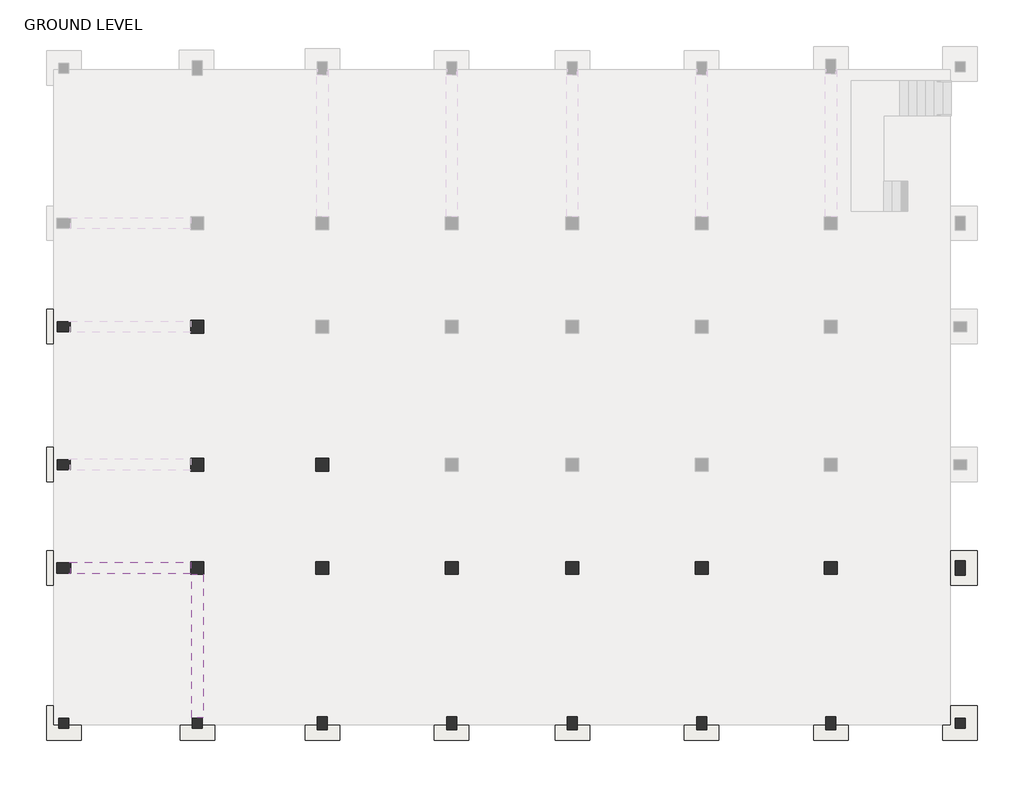
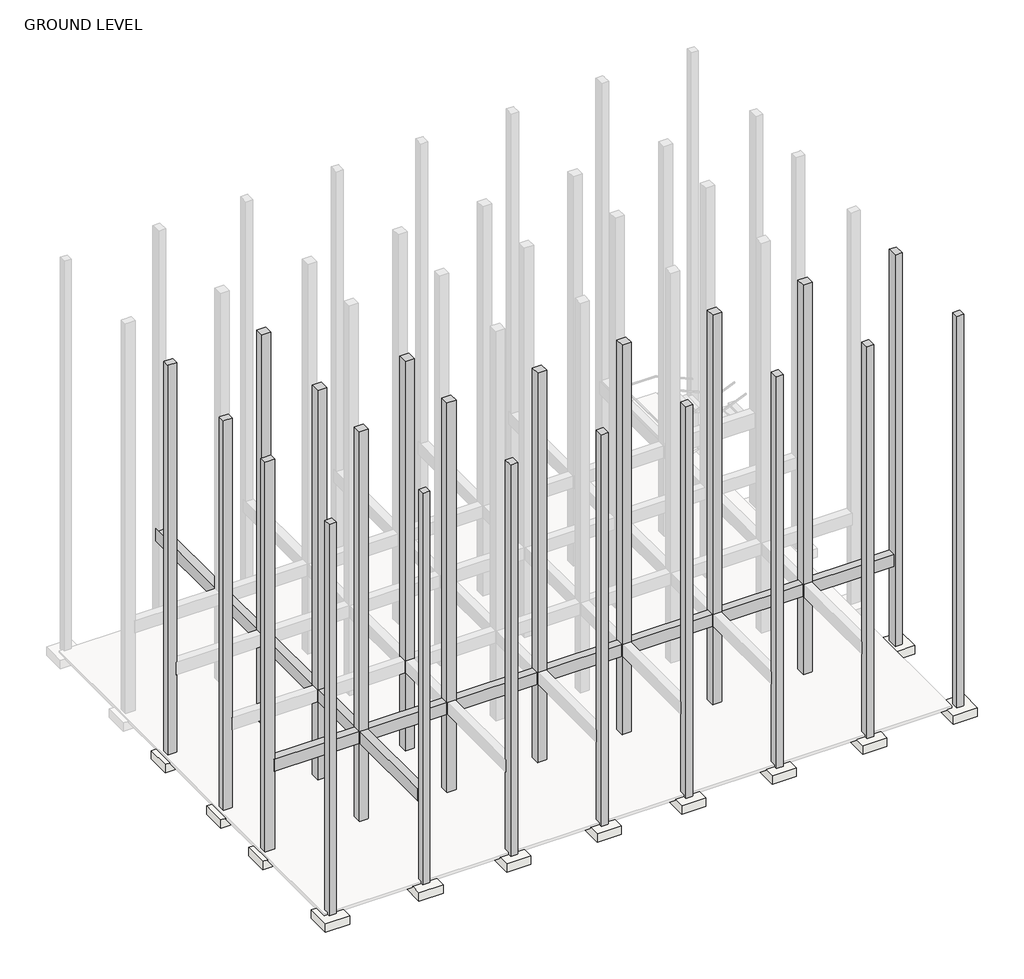
# One storey, part 1 of 3: 21 columns, 21 slabs, 2 beams.
"""IFC4 building model written with IfcOpenShell, lengths in millimetres."""

from ifc_helpers import new_model, si_unit, frame, origin, place, context, project, spatial, polyline, outline, extrude, faceted_brep, element, save

model = new_model("IFC4")

# Units and contexts
model_context = context("Model", 3, world=origin())
ifc_project = project(units=[si_unit("LENGTHUNIT", "METRE", prefix="MILLI")], contexts=[model_context])

# Site, building, storey
site = spatial("IfcSite", under=ifc_project)
building = spatial("IfcBuilding", under=site)
storey = spatial("IfcBuildingStorey", under=building, Name="GROUND LEVEL", Elevation=-1404.4011518)

# Beams
placement = place(None, origin())
element("IfcBeam", 1, ObjectType="M_Concrete-Rectangular Beam : 400 x 800mm", at=placement, inside=storey, context=model_context, shape_type="SweptSolid", body=[
    extrude(outline(polyline([(-20977.1491019, -990.0309165), (-20577.1491019, -990.0309165), (-20577.1491019, -6047.8309165), (-20977.1491019, -6047.8309165), (-20977.1491019, -990.0309165)])), frame((0.0, 0.0, 114.4), z_axis=(0.0, 0.0, 1.0), x_axis=(1.0, 0.0, 0.0)), (0.0, 0.0, 1.0), 647.6),
    extrude(outline(polyline([(-20954.9491019, 16662.9690835), (-20599.3491019, 16662.9690835), (-20599.3491019, 16869.3690835), (-20577.1491019, 16869.3690835), (-20577.1491019, 11659.1690835), (-20977.1491019, 11659.1690835), (-20977.1491019, 16869.3690835), (-20954.9491019, 16869.3690835), (-20954.9491019, 16662.9690835)])), frame((0.0, 0.0, 114.4), z_axis=(0.0, 0.0, 1.0), x_axis=(1.0, 0.0, 0.0)), (0.0, 0.0, 1.0), 647.6),
    extrude(outline(polyline([(-20977.1491019, 11201.9690835), (-20577.1491019, 11201.9690835), (-20577.1491019, 8001.5690835), (-20977.1491019, 8001.5690835), (-20977.1491019, 11201.9690835)])), frame((0.0, 0.0, 114.4), z_axis=(0.0, 0.0, 1.0), x_axis=(1.0, 0.0, 0.0)), (0.0, 0.0, 1.0), 647.6),
    extrude(outline(polyline([(-20977.1491019, 7544.3690835), (-20577.1491019, 7544.3690835), (-20577.1491019, 3124.7690835), (-20977.1491019, 3124.7690835), (-20977.1491019, 7544.3690835)])), frame((0.0, 0.0, 114.4), z_axis=(0.0, 0.0, 1.0), x_axis=(1.0, 0.0, 0.0)), (0.0, 0.0, 1.0), 647.6),
    extrude(outline(polyline([(-20977.1491019, 2667.5690835), (-20577.1491019, 2667.5690835), (-20577.1491019, -532.8309165), (-20977.1491019, -532.8309165), (-20977.1491019, 2667.5690835)])), frame((0.0, 0.0, 114.4), z_axis=(0.0, 0.0, 1.0), x_axis=(1.0, 0.0, 0.0)), (0.0, 0.0, 1.0), 647.6),
])
element("IfcBeam", 2, ObjectType="M_Concrete-Rectangular Beam : 400 x 800mm", at=placement, inside=storey, context=model_context, shape_type="SweptSolid", body=[
    extrude(outline(polyline([(-25247.5491019, -939.2309165), (-25247.5491019, -583.6309165), (-25301.5491019, -583.6309165), (-25301.5491019, -561.4309165), (-21005.7491019, -561.4309165), (-21005.7491019, -961.4309165), (-25301.5491019, -961.4309165), (-25301.5491019, -939.2309165), (-25247.5491019, -939.2309165)])), frame((0.0, 0.0, 114.4), z_axis=(0.0, 0.0, 1.0), x_axis=(1.0, 0.0, 0.0)), (0.0, 0.0, 1.0), 647.6),
    extrude(outline(polyline([(-20548.5491019, -961.4309165), (-20548.5491019, -561.4309165), (-16586.1491019, -561.4309165), (-16586.1491019, -961.4309165), (-20548.5491019, -961.4309165)])), frame((0.0, 0.0, 114.4), z_axis=(0.0, 0.0, 1.0), x_axis=(1.0, 0.0, 0.0)), (0.0, 0.0, 1.0), 647.6),
    extrude(outline(polyline([(-16128.9491019, -961.4309165), (-16128.9491019, -561.4309165), (-12014.1491019, -561.4309165), (-12014.1491019, -961.4309165), (-16128.9491019, -961.4309165)])), frame((0.0, 0.0, 114.4), z_axis=(0.0, 0.0, 1.0), x_axis=(1.0, 0.0, 0.0)), (0.0, 0.0, 1.0), 647.6),
    extrude(outline(polyline([(-11556.9491019, -961.4309165), (-11556.9491019, -561.4309165), (-7746.9491019, -561.4309165), (-7746.9491019, -961.4309165), (-11556.9491019, -961.4309165)])), frame((0.0, 0.0, 114.4), z_axis=(0.0, 0.0, 1.0), x_axis=(1.0, 0.0, 0.0)), (0.0, 0.0, 1.0), 647.6),
    extrude(outline(polyline([(-7289.7491019, -961.4309165), (-7289.7491019, -561.4309165), (-3174.9491019, -561.4309165), (-3174.9491019, -961.4309165), (-7289.7491019, -961.4309165)])), frame((0.0, 0.0, 114.4), z_axis=(0.0, 0.0, 1.0), x_axis=(1.0, 0.0, 0.0)), (0.0, 0.0, 1.0), 647.6),
    extrude(outline(polyline([(-2717.7491019, -961.4309165), (-2717.7491019, -561.4309165), (1397.0508981, -561.4309165), (1397.0508981, -961.4309165), (-2717.7491019, -961.4309165)])), frame((0.0, 0.0, 114.4), z_axis=(0.0, 0.0, 1.0), x_axis=(1.0, 0.0, 0.0)), (0.0, 0.0, 1.0), 647.6),
    extrude(outline(polyline([(1854.2508981, -961.4309165), (1854.2508981, -561.4309165), (5997.6508981, -561.4309165), (5997.6508981, -961.4309165), (1854.2508981, -961.4309165)])), frame((0.0, 0.0, 114.4), z_axis=(0.0, 0.0, 1.0), x_axis=(1.0, 0.0, 0.0)), (0.0, 0.0, 1.0), 647.6),
])

# Columns
element("IfcColumn", 3, ObjectType="M_Concrete-Rectangular-Column : C1", at=placement, inside=storey, context=model_context, shape_type="SweptSolid", body=[
    extrude(outline(polyline([(-25323.7491019, -6070.0309165), (-25323.7491019, -6425.6309165), (-25679.3491019, -6425.6309165), (-25679.3491019, -6070.0309165), (-25323.7491019, -6070.0309165)])), frame((0.0, 0.0, -4147.6011518), z_axis=(0.0, 0.0, 1.0), x_axis=(1.0, 0.0, 0.0)), (0.0, 0.0, 1.0), 20911.6011518),
])
element("IfcColumn", 4, ObjectType="M_Concrete-Rectangular-Column : C1", at=placement, inside=storey, context=model_context, shape_type="Brep", body=[
    faceted_brep([(-20599.3491019, -6070.0309165, -4147.6011518), (-20599.3491019, -6425.6309165, -4147.6011518), (-20954.9491019, -6425.6309165, -4147.6011518), (-20954.9491019, -6070.0309165, -4147.6011518), (-20599.3491019, -6070.0309165, 16764.0), (-20599.3491019, -6425.6309165, 16764.0), (-20599.3491019, -6425.6309165, 16611.6), (-20599.3491019, -6425.6309165, 15964.0), (-20599.3491019, -6425.6309165, 13563.6), (-20599.3491019, -6425.6309165, 12916.0), (-20599.3491019, -6425.6309165, 10515.6), (-20599.3491019, -6425.6309165, 9868.0), (-20599.3491019, -6425.6309165, 7467.6), (-20599.3491019, -6425.6309165, 6820.0), (-20599.3491019, -6425.6309165, 4419.6), (-20599.3491019, -6425.6309165, 3772.0), (-20599.3491019, -6425.6309165, 762.0), (-20599.3491019, -6425.6309165, 114.4), (-20599.3491019, -6070.0309165, 114.4), (-20599.3491019, -6070.0309165, 762.0), (-20599.3491019, -6070.0309165, 3772.0), (-20599.3491019, -6070.0309165, 4419.6), (-20599.3491019, -6070.0309165, 6820.0), (-20599.3491019, -6070.0309165, 7467.6), (-20599.3491019, -6070.0309165, 9868.0), (-20599.3491019, -6070.0309165, 10515.6), (-20599.3491019, -6070.0309165, 12916.0), (-20599.3491019, -6070.0309165, 13563.6), (-20599.3491019, -6070.0309165, 15964.0), (-20599.3491019, -6070.0309165, 16611.6), (-20954.9491019, -6425.6309165, 16764.0), (-20954.9491019, -6425.6309165, 16611.6), (-20954.9491019, -6425.6309165, 15964.0), (-20954.9491019, -6425.6309165, 13563.6), (-20954.9491019, -6425.6309165, 12916.0), (-20954.9491019, -6425.6309165, 10515.6), (-20954.9491019, -6425.6309165, 9868.0), (-20954.9491019, -6425.6309165, 7467.6), (-20954.9491019, -6425.6309165, 6820.0), (-20954.9491019, -6425.6309165, 4419.6), (-20954.9491019, -6425.6309165, 3772.0), (-20954.9491019, -6425.6309165, 762.0), (-20954.9491019, -6425.6309165, 114.4), (-20954.9491019, -6070.0309165, 16764.0), (-20954.9491019, -6070.0309165, 16611.6), (-20954.9491019, -6070.0309165, 15964.0), (-20954.9491019, -6070.0309165, 13563.6), (-20954.9491019, -6070.0309165, 12916.0), (-20954.9491019, -6070.0309165, 10515.6), (-20954.9491019, -6070.0309165, 9868.0), (-20954.9491019, -6070.0309165, 7467.6), (-20954.9491019, -6070.0309165, 6820.0), (-20954.9491019, -6070.0309165, 4419.6), (-20954.9491019, -6070.0309165, 3772.0), (-20954.9491019, -6070.0309165, 762.0), (-20954.9491019, -6070.0309165, 114.4)], [[[0, 1, 2, 3]], [[4, 5, 6, 7, 8, 9, 10, 11, 12, 13, 14, 15, 16, 17, 1, 0, 18, 19, 20, 21, 22, 23, 24, 25, 26, 27, 28, 29]], [[5, 30, 31, 32, 33, 34, 35, 36, 37, 38, 39, 40, 41, 42, 2, 1, 17, 16, 15, 14, 13, 12, 11, 10, 9, 8, 7, 6]], [[30, 43, 44, 45, 46, 47, 48, 49, 50, 51, 52, 53, 54, 55, 3, 2, 42, 41, 40, 39, 38, 37, 36, 35, 34, 33, 32, 31]], [[43, 4, 29, 28, 27, 26, 25, 24, 23, 22, 21, 20, 19, 18, 0, 3, 55, 54, 53, 52, 51, 50, 49, 48, 47, 46, 45, 44]], [[4, 43, 30, 5]]]),
])
element("IfcColumn", 5, ObjectType="M_Concrete-Rectangular-Column : C1", at=placement, inside=storey, context=model_context, shape_type="SweptSolid", body=[
    extrude(outline(polyline([(6375.4508981, -6070.0309165), (6375.4508981, -6425.6309165), (6019.8508981, -6425.6309165), (6019.8508981, -6070.0309165), (6375.4508981, -6070.0309165)])), frame((0.0, 0.0, -4147.6011518), z_axis=(0.0, 0.0, 1.0), x_axis=(1.0, 0.0, 0.0)), (0.0, 0.0, 1.0), 20911.6011518),
])
element("IfcColumn", 6, ObjectType="M_Concrete-Rectangular-Column : C2", at=placement, inside=storey, context=model_context, shape_type="Brep", body=[
    faceted_brep([(-25730.1491019, 7950.7690835, -4147.6011518), (-25272.9491019, 7950.7690835, -4147.6011518), (-25272.9491019, 7595.1690835, -4147.6011518), (-25730.1491019, 7595.1690835, -4147.6011518), (-25730.1491019, 7950.7690835, 16764.0), (-25701.5491019, 7950.7690835, 16764.0), (-25679.3491019, 7950.7690835, 16764.0), (-25272.9491019, 7950.7690835, 16764.0), (-25272.9491019, 7595.1690835, 16764.0), (-25679.3491019, 7595.1690835, 16764.0), (-25701.5491019, 7595.1690835, 16764.0), (-25730.1491019, 7595.1690835, 16764.0)], [[[0, 1, 2, 3]], [[4, 5, 6, 7, 1, 0]], [[7, 8, 2, 1]], [[8, 9, 10, 11, 3, 2]], [[11, 4, 0, 3]], [[4, 11, 10, 9, 8, 7, 6, 5]]]),
])
element("IfcColumn", 7, ObjectType="M_Concrete-Rectangular-Column : C2", at=placement, inside=storey, context=model_context, shape_type="Brep", body=[
    faceted_brep([(-25730.1491019, 3073.9690835, -4147.6011518), (-25272.9491019, 3073.9690835, -4147.6011518), (-25272.9491019, 2718.3690835, -4147.6011518), (-25730.1491019, 2718.3690835, -4147.6011518), (-25730.1491019, 3073.9690835, 16764.0), (-25701.5491019, 3073.9690835, 16764.0), (-25679.3491019, 3073.9690835, 16764.0), (-25272.9491019, 3073.9690835, 16764.0), (-25272.9491019, 2718.3690835, 16764.0), (-25679.3491019, 2718.3690835, 16764.0), (-25701.5491019, 2718.3690835, 16764.0), (-25730.1491019, 2718.3690835, 16764.0)], [[[0, 1, 2, 3]], [[4, 5, 6, 7, 1, 0]], [[7, 8, 2, 1]], [[8, 9, 10, 11, 3, 2]], [[11, 4, 0, 3]], [[4, 11, 10, 9, 8, 7, 6, 5]]]),
])
element("IfcColumn", 8, ObjectType="M_Concrete-Rectangular-Column : C2", at=placement, inside=storey, context=model_context, shape_type="Brep", body=[
    faceted_brep([(-16179.7491019, -6019.2309165, -4147.6011518), (-16179.7491019, -6476.4309165, -4147.6011518), (-16535.3491019, -6476.4309165, -4147.6011518), (-16535.3491019, -6019.2309165, -4147.6011518), (-16179.7491019, -6019.2309165, 16764.0), (-16179.7491019, -6425.6309165, 16764.0), (-16179.7491019, -6447.8309165, 16764.0), (-16179.7491019, -6476.4309165, 16764.0), (-16535.3491019, -6476.4309165, 16764.0), (-16535.3491019, -6447.8309165, 16764.0), (-16535.3491019, -6425.6309165, 16764.0), (-16535.3491019, -6019.2309165, 16764.0)], [[[0, 1, 2, 3]], [[4, 5, 6, 7, 1, 0]], [[7, 8, 2, 1]], [[8, 9, 10, 11, 3, 2]], [[11, 4, 0, 3]], [[4, 11, 10, 9, 8, 7, 6, 5]]]),
])
element("IfcColumn", 9, ObjectType="M_Concrete-Rectangular-Column : C2", at=placement, inside=storey, context=model_context, shape_type="Brep", body=[
    faceted_brep([(-11607.7491019, -6019.2309165, -4147.6011518), (-11607.7491019, -6476.4309165, -4147.6011518), (-11963.3491019, -6476.4309165, -4147.6011518), (-11963.3491019, -6019.2309165, -4147.6011518), (-11607.7491019, -6019.2309165, 16764.0), (-11607.7491019, -6425.6309165, 16764.0), (-11607.7491019, -6447.8309165, 16764.0), (-11607.7491019, -6476.4309165, 16764.0), (-11963.3491019, -6476.4309165, 16764.0), (-11963.3491019, -6447.8309165, 16764.0), (-11963.3491019, -6425.6309165, 16764.0), (-11963.3491019, -6019.2309165, 16764.0)], [[[0, 1, 2, 3]], [[4, 5, 6, 7, 1, 0]], [[7, 8, 2, 1]], [[8, 9, 10, 11, 3, 2]], [[11, 4, 0, 3]], [[4, 11, 10, 9, 8, 7, 6, 5]]]),
])
element("IfcColumn", 10, ObjectType="M_Concrete-Rectangular-Column : C2", at=placement, inside=storey, context=model_context, shape_type="Brep", body=[
    faceted_brep([(-7340.5491019, -6019.2309165, -4147.6011518), (-7340.5491019, -6476.4309165, -4147.6011518), (-7696.1491019, -6476.4309165, -4147.6011518), (-7696.1491019, -6019.2309165, -4147.6011518), (-7340.5491019, -6019.2309165, 16764.0), (-7340.5491019, -6425.6309165, 16764.0), (-7340.5491019, -6447.8309165, 16764.0), (-7340.5491019, -6476.4309165, 16764.0), (-7696.1491019, -6476.4309165, 16764.0), (-7696.1491019, -6447.8309165, 16764.0), (-7696.1491019, -6425.6309165, 16764.0), (-7696.1491019, -6019.2309165, 16764.0)], [[[0, 1, 2, 3]], [[4, 5, 6, 7, 1, 0]], [[7, 8, 2, 1]], [[8, 9, 10, 11, 3, 2]], [[11, 4, 0, 3]], [[4, 11, 10, 9, 8, 7, 6, 5]]]),
])
element("IfcColumn", 11, ObjectType="M_Concrete-Rectangular-Column : C2", at=placement, inside=storey, context=model_context, shape_type="Brep", body=[
    faceted_brep([(-2768.5491019, -6019.2309165, -4147.6011518), (-2768.5491019, -6476.4309165, -4147.6011518), (-3124.1491019, -6476.4309165, -4147.6011518), (-3124.1491019, -6019.2309165, -4147.6011518), (-2768.5491019, -6019.2309165, 16764.0), (-2768.5491019, -6425.6309165, 16764.0), (-2768.5491019, -6447.8309165, 16764.0), (-2768.5491019, -6476.4309165, 16764.0), (-3124.1491019, -6476.4309165, 16764.0), (-3124.1491019, -6447.8309165, 16764.0), (-3124.1491019, -6425.6309165, 16764.0), (-3124.1491019, -6019.2309165, 16764.0)], [[[0, 1, 2, 3]], [[4, 5, 6, 7, 1, 0]], [[7, 8, 2, 1]], [[8, 9, 10, 11, 3, 2]], [[11, 4, 0, 3]], [[4, 11, 10, 9, 8, 7, 6, 5]]]),
])
element("IfcColumn", 12, ObjectType="M_Concrete-Rectangular-Column : C2", at=placement, inside=storey, context=model_context, shape_type="Brep", body=[
    faceted_brep([(1803.4508981, -6019.2309165, -4147.6011518), (1803.4508981, -6476.4309165, -4147.6011518), (1447.8508981, -6476.4309165, -4147.6011518), (1447.8508981, -6019.2309165, -4147.6011518), (1803.4508981, -6019.2309165, 16764.0), (1803.4508981, -6425.6309165, 16764.0), (1803.4508981, -6447.8309165, 16764.0), (1803.4508981, -6476.4309165, 16764.0), (1447.8508981, -6476.4309165, 16764.0), (1447.8508981, -6447.8309165, 16764.0), (1447.8508981, -6425.6309165, 16764.0), (1447.8508981, -6019.2309165, 16764.0)], [[[0, 1, 2, 3]], [[4, 5, 6, 7, 1, 0]], [[7, 8, 2, 1]], [[8, 9, 10, 11, 3, 2]], [[11, 4, 0, 3]], [[4, 11, 10, 9, 8, 7, 6, 5]]]),
])
element("IfcColumn", 13, ObjectType="M_Concrete-Rectangular-Column : C3", at=placement, inside=storey, context=model_context, shape_type="SweptSolid", body=[
    extrude(outline(polyline([(-20548.5491019, 8001.5690835), (-20548.5491019, 7544.3690835), (-21005.7491019, 7544.3690835), (-21005.7491019, 8001.5690835), (-20548.5491019, 8001.5690835)])), frame((0.0, 0.0, -4147.6011518), z_axis=(0.0, 0.0, 1.0), x_axis=(1.0, 0.0, 0.0)), (0.0, 0.0, 1.0), 20911.6011518),
])
element("IfcColumn", 14, ObjectType="M_Concrete-Rectangular-Column : C3", at=placement, inside=storey, context=model_context, shape_type="SweptSolid", body=[
    extrude(outline(polyline([(-20548.5491019, 3124.7690835), (-20548.5491019, 2667.5690835), (-21005.7491019, 2667.5690835), (-21005.7491019, 3124.7690835), (-20548.5491019, 3124.7690835)])), frame((0.0, 0.0, -4147.6011518), z_axis=(0.0, 0.0, 1.0), x_axis=(1.0, 0.0, 0.0)), (0.0, 0.0, 1.0), 20911.6011518),
])
element("IfcColumn", 15, ObjectType="M_Concrete-Rectangular-Column : C3", at=placement, inside=storey, context=model_context, shape_type="SweptSolid", body=[
    extrude(outline(polyline([(-16128.9491019, 3124.7690835), (-16128.9491019, 2667.5690835), (-16586.1491019, 2667.5690835), (-16586.1491019, 3124.7690835), (-16128.9491019, 3124.7690835)])), frame((0.0, 0.0, -4147.6011518), z_axis=(0.0, 0.0, 1.0), x_axis=(1.0, 0.0, 0.0)), (0.0, 0.0, 1.0), 20911.6011518),
])
element("IfcColumn", 16, ObjectType="M_Concrete-Rectangular-Column : C3", at=placement, inside=storey, context=model_context, shape_type="SweptSolid", body=[
    extrude(outline(polyline([(-20548.5491019, -532.8309165), (-20548.5491019, -990.0309165), (-21005.7491019, -990.0309165), (-21005.7491019, -532.8309165), (-20548.5491019, -532.8309165)])), frame((0.0, 0.0, -4147.6011518), z_axis=(0.0, 0.0, 1.0), x_axis=(1.0, 0.0, 0.0)), (0.0, 0.0, 1.0), 20911.6011518),
])
element("IfcColumn", 17, ObjectType="M_Concrete-Rectangular-Column : C3", at=placement, inside=storey, context=model_context, shape_type="SweptSolid", body=[
    extrude(outline(polyline([(-16128.9491019, -532.8309165), (-16128.9491019, -990.0309165), (-16586.1491019, -990.0309165), (-16586.1491019, -532.8309165), (-16128.9491019, -532.8309165)])), frame((0.0, 0.0, -4147.6011518), z_axis=(0.0, 0.0, 1.0), x_axis=(1.0, 0.0, 0.0)), (0.0, 0.0, 1.0), 20911.6011518),
])
element("IfcColumn", 18, ObjectType="M_Concrete-Rectangular-Column : C3", at=placement, inside=storey, context=model_context, shape_type="SweptSolid", body=[
    extrude(outline(polyline([(-11556.9491019, -532.8309165), (-11556.9491019, -990.0309165), (-12014.1491019, -990.0309165), (-12014.1491019, -532.8309165), (-11556.9491019, -532.8309165)])), frame((0.0, 0.0, -4147.6011518), z_axis=(0.0, 0.0, 1.0), x_axis=(1.0, 0.0, 0.0)), (0.0, 0.0, 1.0), 20911.6011518),
])
element("IfcColumn", 19, ObjectType="M_Concrete-Rectangular-Column : C3", at=placement, inside=storey, context=model_context, shape_type="SweptSolid", body=[
    extrude(outline(polyline([(-7289.7491019, -532.8309165), (-7289.7491019, -990.0309165), (-7746.9491019, -990.0309165), (-7746.9491019, -532.8309165), (-7289.7491019, -532.8309165)])), frame((0.0, 0.0, -4147.6011518), z_axis=(0.0, 0.0, 1.0), x_axis=(1.0, 0.0, 0.0)), (0.0, 0.0, 1.0), 20911.6011518),
])
element("IfcColumn", 20, ObjectType="M_Concrete-Rectangular-Column : C3", at=placement, inside=storey, context=model_context, shape_type="SweptSolid", body=[
    extrude(outline(polyline([(-2717.7491019, -532.8309165), (-2717.7491019, -990.0309165), (-3174.9491019, -990.0309165), (-3174.9491019, -532.8309165), (-2717.7491019, -532.8309165)])), frame((0.0, 0.0, -4147.6011518), z_axis=(0.0, 0.0, 1.0), x_axis=(1.0, 0.0, 0.0)), (0.0, 0.0, 1.0), 20911.6011518),
])
element("IfcColumn", 21, ObjectType="M_Concrete-Rectangular-Column : C3", at=placement, inside=storey, context=model_context, shape_type="SweptSolid", body=[
    extrude(outline(polyline([(1854.2508981, -532.8309165), (1854.2508981, -990.0309165), (1397.0508981, -990.0309165), (1397.0508981, -532.8309165), (1854.2508981, -532.8309165)])), frame((0.0, 0.0, -4147.6011518), z_axis=(0.0, 0.0, 1.0), x_axis=(1.0, 0.0, 0.0)), (0.0, 0.0, 1.0), 20911.6011518),
])
element("IfcColumn", 22, ObjectType="M_Concrete-Rectangular-Column : C4", at=placement, inside=storey, context=model_context, shape_type="Brep", body=[
    faceted_brep([(6375.4508981, -507.4309165, -4147.6011518), (6375.4508981, -1015.4309165, -4147.6011518), (6019.8508981, -1015.4309165, -4147.6011518), (6019.8508981, -507.4309165, -4147.6011518), (6375.4508981, -507.4309165, 16764.0), (6375.4508981, -1015.4309165, 16764.0), (6375.4508981, -1015.4309165, 16611.6), (6375.4508981, -1015.4309165, 15964.0), (6375.4508981, -1015.4309165, 13563.6), (6375.4508981, -1015.4309165, 12916.0), (6375.4508981, -1015.4309165, 10515.6), (6375.4508981, -1015.4309165, 9868.0), (6375.4508981, -1015.4309165, 7467.6), (6375.4508981, -1015.4309165, 6820.0), (6375.4508981, -1015.4309165, 4419.6), (6375.4508981, -1015.4309165, 3772.0), (6375.4508981, -1015.4309165, 762.0), (6375.4508981, -1015.4309165, 114.4), (6375.4508981, -507.4309165, 114.4), (6375.4508981, -507.4309165, 762.0), (6375.4508981, -507.4309165, 3772.0), (6375.4508981, -507.4309165, 4419.6), (6375.4508981, -507.4309165, 6820.0), (6375.4508981, -507.4309165, 7467.6), (6375.4508981, -507.4309165, 9868.0), (6375.4508981, -507.4309165, 10515.6), (6375.4508981, -507.4309165, 12916.0), (6375.4508981, -507.4309165, 13563.6), (6375.4508981, -507.4309165, 15964.0), (6375.4508981, -507.4309165, 16611.6), (6019.8508981, -1015.4309165, 16764.0), (6019.8508981, -1015.4309165, 16611.6), (6019.8508981, -1015.4309165, 15964.0), (6019.8508981, -1015.4309165, 13563.6), (6019.8508981, -1015.4309165, 12916.0), (6019.8508981, -1015.4309165, 10515.6), (6019.8508981, -1015.4309165, 9868.0), (6019.8508981, -1015.4309165, 7467.6), (6019.8508981, -1015.4309165, 6820.0), (6019.8508981, -1015.4309165, 4419.6), (6019.8508981, -1015.4309165, 3772.0), (6019.8508981, -1015.4309165, 762.0), (6019.8508981, -1015.4309165, 114.4), (6019.8508981, -507.4309165, 16764.0), (6019.8508981, -507.4309165, 16611.6), (6019.8508981, -507.4309165, 15964.0), (6019.8508981, -507.4309165, 13563.6), (6019.8508981, -507.4309165, 12916.0), (6019.8508981, -507.4309165, 10515.6), (6019.8508981, -507.4309165, 9868.0), (6019.8508981, -507.4309165, 7467.6), (6019.8508981, -507.4309165, 6820.0), (6019.8508981, -507.4309165, 4419.6), (6019.8508981, -507.4309165, 3772.0), (6019.8508981, -507.4309165, 762.0), (6019.8508981, -507.4309165, 114.4)], [[[0, 1, 2, 3]], [[4, 5, 6, 7, 8, 9, 10, 11, 12, 13, 14, 15, 16, 17, 1, 0, 18, 19, 20, 21, 22, 23, 24, 25, 26, 27, 28, 29]], [[5, 30, 31, 32, 33, 34, 35, 36, 37, 38, 39, 40, 41, 42, 2, 1, 17, 16, 15, 14, 13, 12, 11, 10, 9, 8, 7, 6]], [[30, 43, 44, 45, 46, 47, 48, 49, 50, 51, 52, 53, 54, 55, 3, 2, 42, 41, 40, 39, 38, 37, 36, 35, 34, 33, 32, 31]], [[43, 4, 29, 28, 27, 26, 25, 24, 23, 22, 21, 20, 19, 18, 0, 3, 55, 54, 53, 52, 51, 50, 49, 48, 47, 46, 45, 44]], [[4, 43, 30, 5]]]),
])
element("IfcColumn", 23, ObjectType="M_Concrete-Rectangular-Column : C4", at=placement, inside=storey, context=model_context, shape_type="Brep", body=[
    faceted_brep([(-25755.5491019, -583.6309165, -4147.6011518), (-25247.5491019, -583.6309165, -4147.6011518), (-25247.5491019, -939.2309165, -4147.6011518), (-25755.5491019, -939.2309165, -4147.6011518), (-25755.5491019, -583.6309165, 16764.0), (-25701.5491019, -583.6309165, 16764.0), (-25679.3491019, -583.6309165, 16764.0), (-25247.5491019, -583.6309165, 16764.0), (-25247.5491019, -939.2309165, 16764.0), (-25679.3491019, -939.2309165, 16764.0), (-25701.5491019, -939.2309165, 16764.0), (-25755.5491019, -939.2309165, 16764.0)], [[[0, 1, 2, 3]], [[4, 5, 6, 7, 1, 0]], [[7, 8, 2, 1]], [[8, 9, 10, 11, 3, 2]], [[11, 4, 0, 3]], [[4, 11, 10, 9, 8, 7, 6, 5]]]),
])

# Slabs
element("IfcSlab", 24, ObjectType="M_Footing-Rectangular : F 5", at=placement, inside=storey, context=model_context, shape_type="SweptSolid", body=[
    extrude(outline(polyline([(-4597.6011518, -26111.1491019), (-4597.6011518, -24891.9491019), (-4197.8282159, -24891.9491019), (-4197.8282159, -25857.1491019), (-4147.6011518, -25857.1491019), (-4147.6011518, -26111.1491019), (-4597.6011518, -26111.1491019)])), frame((0.0, 7163.3690835, 0.0), z_axis=(0.0, 1.0, 0.0), x_axis=(0.0, 0.0, 1.0)), (0.0, 0.0, 1.0), 1219.2),
])
element("IfcSlab", 25, ObjectType="M_Footing-Rectangular : F 5", at=placement, inside=storey, context=model_context, shape_type="SweptSolid", body=[
    extrude(outline(polyline([(-20167.5491019, 8382.5690835), (-20167.5491019, 7163.3690835), (-21386.7491019, 7163.3690835), (-21386.7491019, 8382.5690835), (-20167.5491019, 8382.5690835)])), frame((0.0, 0.0, -4597.6011518), z_axis=(0.0, 0.0, 1.0), x_axis=(1.0, 0.0, 0.0)), (0.0, 0.0, 1.0), 399.772936),
])
element("IfcSlab", 26, ObjectType="M_Footing-Rectangular : F 5", at=placement, inside=storey, context=model_context, shape_type="SweptSolid", body=[
    extrude(outline(polyline([(-15747.9491019, 3505.7690835), (-15747.9491019, 2286.5690835), (-16967.1491019, 2286.5690835), (-16967.1491019, 3505.7690835), (-15747.9491019, 3505.7690835)])), frame((0.0, 0.0, -4597.6011518), z_axis=(0.0, 0.0, 1.0), x_axis=(1.0, 0.0, 0.0)), (0.0, 0.0, 1.0), 399.772936),
])
element("IfcSlab", 27, ObjectType="M_Footing-Rectangular : F 5", at=placement, inside=storey, context=model_context, shape_type="SweptSolid", body=[
    extrude(outline(polyline([(-20167.5491019, 3505.7690835), (-20167.5491019, 2286.5690835), (-21386.7491019, 2286.5690835), (-21386.7491019, 3505.7690835), (-20167.5491019, 3505.7690835)])), frame((0.0, 0.0, -4597.6011518), z_axis=(0.0, 0.0, 1.0), x_axis=(1.0, 0.0, 0.0)), (0.0, 0.0, 1.0), 399.772936),
])
element("IfcSlab", 28, ObjectType="M_Footing-Rectangular : F 5", at=placement, inside=storey, context=model_context, shape_type="SweptSolid", body=[
    extrude(outline(polyline([(-4597.6011518, -26111.1491019), (-4597.6011518, -24891.9491019), (-4197.8282159, -24891.9491019), (-4197.8282159, -25857.1491019), (-4147.6011518, -25857.1491019), (-4147.6011518, -26111.1491019), (-4597.6011518, -26111.1491019)])), frame((0.0, 2286.5690835, 0.0), z_axis=(0.0, 1.0, 0.0), x_axis=(0.0, 0.0, 1.0)), (0.0, 0.0, 1.0), 1219.2),
])
element("IfcSlab", 29, ObjectType="M_Footing-Rectangular : F 5", at=placement, inside=storey, context=model_context, shape_type="SweptSolid", body=[
    extrude(outline(polyline([(-4597.6011518, -26111.1491019), (-4597.6011518, -24891.9491019), (-4197.8282159, -24891.9491019), (-4197.8282159, -25857.1491019), (-4147.6011518, -25857.1491019), (-4147.6011518, -26111.1491019), (-4597.6011518, -26111.1491019)])), frame((0.0, -1371.0309165, 0.0), z_axis=(0.0, 1.0, 0.0), x_axis=(0.0, 0.0, 1.0)), (0.0, 0.0, 1.0), 1219.2),
])
element("IfcSlab", 30, ObjectType="M_Footing-Rectangular : F 5", at=placement, inside=storey, context=model_context, shape_type="SweptSolid", body=[
    extrude(outline(polyline([(-20167.5491019, -151.8309165), (-20167.5491019, -1371.0309165), (-21386.7491019, -1371.0309165), (-21386.7491019, -151.8309165), (-20167.5491019, -151.8309165)])), frame((0.0, 0.0, -4597.6011518), z_axis=(0.0, 0.0, 1.0), x_axis=(1.0, 0.0, 0.0)), (0.0, 0.0, 1.0), 399.772936),
])
element("IfcSlab", 31, ObjectType="M_Footing-Rectangular : F 5", at=placement, inside=storey, context=model_context, shape_type="SweptSolid", body=[
    extrude(outline(polyline([(-15747.9491019, -151.8309165), (-15747.9491019, -1371.0309165), (-16967.1491019, -1371.0309165), (-16967.1491019, -151.8309165), (-15747.9491019, -151.8309165)])), frame((0.0, 0.0, -4597.6011518), z_axis=(0.0, 0.0, 1.0), x_axis=(1.0, 0.0, 0.0)), (0.0, 0.0, 1.0), 399.772936),
])
element("IfcSlab", 32, ObjectType="M_Footing-Rectangular : F 5", at=placement, inside=storey, context=model_context, shape_type="SweptSolid", body=[
    extrude(outline(polyline([(-11175.9491019, -151.8309165), (-11175.9491019, -1371.0309165), (-12395.1491019, -1371.0309165), (-12395.1491019, -151.8309165), (-11175.9491019, -151.8309165)])), frame((0.0, 0.0, -4597.6011518), z_axis=(0.0, 0.0, 1.0), x_axis=(1.0, 0.0, 0.0)), (0.0, 0.0, 1.0), 399.772936),
])
element("IfcSlab", 33, ObjectType="M_Footing-Rectangular : F 5", at=placement, inside=storey, context=model_context, shape_type="SweptSolid", body=[
    extrude(outline(polyline([(-6908.7491019, -151.8309165), (-6908.7491019, -1371.0309165), (-8127.9491019, -1371.0309165), (-8127.9491019, -151.8309165), (-6908.7491019, -151.8309165)])), frame((0.0, 0.0, -4597.6011518), z_axis=(0.0, 0.0, 1.0), x_axis=(1.0, 0.0, 0.0)), (0.0, 0.0, 1.0), 399.772936),
])
element("IfcSlab", 34, ObjectType="M_Footing-Rectangular : F 5", at=placement, inside=storey, context=model_context, shape_type="SweptSolid", body=[
    extrude(outline(polyline([(-2336.7491019, -151.8309165), (-2336.7491019, -1371.0309165), (-3555.9491019, -1371.0309165), (-3555.9491019, -151.8309165), (-2336.7491019, -151.8309165)])), frame((0.0, 0.0, -4597.6011518), z_axis=(0.0, 0.0, 1.0), x_axis=(1.0, 0.0, 0.0)), (0.0, 0.0, 1.0), 399.772936),
])
element("IfcSlab", 35, ObjectType="M_Footing-Rectangular : F 5", at=placement, inside=storey, context=model_context, shape_type="SweptSolid", body=[
    extrude(outline(polyline([(2235.2508981, -151.8309165), (2235.2508981, -1371.0309165), (1016.0508981, -1371.0309165), (1016.0508981, -151.8309165), (2235.2508981, -151.8309165)])), frame((0.0, 0.0, -4597.6011518), z_axis=(0.0, 0.0, 1.0), x_axis=(1.0, 0.0, 0.0)), (0.0, 0.0, 1.0), 399.772936),
])
element("IfcSlab", 36, ObjectType="M_Footing-Rectangular : F 5", at=placement, inside=storey, context=model_context, shape_type="SweptSolid", body=[
    extrude(outline(polyline([(-4597.6011518, 5588.0508981), (-4597.6011518, 6807.2508981), (-4147.6011518, 6807.2508981), (-4147.6011518, 5842.0508981), (-4197.8282159, 5842.0508981), (-4197.8282159, 5588.0508981), (-4597.6011518, 5588.0508981)])), frame((0.0, -1371.0309165, 0.0), z_axis=(0.0, 1.0, 0.0), x_axis=(0.0, 0.0, 1.0)), (0.0, 0.0, 1.0), 1219.2),
])
element("IfcSlab", 37, ObjectType="M_Footing-Rectangular : F 5", at=placement, inside=storey, context=model_context, shape_type="Brep", body=[
    faceted_brep([(5588.0508981, -6857.4309165, -4147.6011518), (6807.2508981, -6857.4309165, -4147.6011518), (6807.2508981, -5638.2309165, -4147.6011518), (5842.0508981, -5638.2309165, -4147.6011518), (5842.0508981, -6302.8455236, -4147.6011518), (5588.0508981, -6302.8455236, -4147.6011518), (6807.2508981, -5638.2309165, -4597.6011518), (6807.2508981, -6857.4309165, -4597.6011518), (5588.0508981, -6857.4309165, -4597.6011518), (5588.0508981, -5638.2309165, -4597.6011518), (5588.0508981, -5638.2309165, -4197.8282159), (5842.0508981, -5638.2309165, -4197.8282159), (5588.0508981, -6302.8455236, -4197.8282159), (5842.0508981, -6302.8455236, -4197.8282159)], [[[0, 1, 2, 3, 4, 5]], [[6, 7, 8, 9]], [[6, 9, 10, 11, 3, 2]], [[9, 8, 0, 5, 12, 10]], [[1, 0, 8, 7]], [[2, 1, 7, 6]], [[12, 13, 11, 10]], [[11, 13, 4, 3]], [[13, 12, 5, 4]]]),
])
element("IfcSlab", 38, ObjectType="M_Footing-Rectangular : F 5", at=placement, inside=storey, context=model_context, shape_type="SweptSolid", body=[
    extrude(outline(polyline([(-5638.2309165, -4597.6011518), (-6857.4309165, -4597.6011518), (-6857.4309165, -4147.6011518), (-6302.8455236, -4147.6011518), (-6302.8455236, -4197.8282159), (-5638.2309165, -4197.8282159), (-5638.2309165, -4597.6011518)])), frame((1016.0508981, 0.0, 0.0), z_axis=(1.0, 0.0, 0.0), x_axis=(0.0, 1.0, 0.0)), (0.0, 0.0, 1.0), 1219.2),
])
element("IfcSlab", 39, ObjectType="M_Footing-Rectangular : F 5", at=placement, inside=storey, context=model_context, shape_type="SweptSolid", body=[
    extrude(outline(polyline([(-5638.2309165, -4597.6011518), (-6857.4309165, -4597.6011518), (-6857.4309165, -4147.6011518), (-6302.8455236, -4147.6011518), (-6302.8455236, -4197.8282159), (-5638.2309165, -4197.8282159), (-5638.2309165, -4597.6011518)])), frame((-3555.9491019, 0.0, 0.0), z_axis=(1.0, 0.0, 0.0), x_axis=(0.0, 1.0, 0.0)), (0.0, 0.0, 1.0), 1219.2),
])
element("IfcSlab", 40, ObjectType="M_Footing-Rectangular : F 5", at=placement, inside=storey, context=model_context, shape_type="SweptSolid", body=[
    extrude(outline(polyline([(-5638.2309165, -4597.6011518), (-6857.4309165, -4597.6011518), (-6857.4309165, -4147.6011518), (-6302.8455236, -4147.6011518), (-6302.8455236, -4197.8282159), (-5638.2309165, -4197.8282159), (-5638.2309165, -4597.6011518)])), frame((-8127.9491019, 0.0, 0.0), z_axis=(1.0, 0.0, 0.0), x_axis=(0.0, 1.0, 0.0)), (0.0, 0.0, 1.0), 1219.2),
])
element("IfcSlab", 41, ObjectType="M_Footing-Rectangular : F 5", at=placement, inside=storey, context=model_context, shape_type="SweptSolid", body=[
    extrude(outline(polyline([(-5638.2309165, -4597.6011518), (-6857.4309165, -4597.6011518), (-6857.4309165, -4147.6011518), (-6302.8455236, -4147.6011518), (-6302.8455236, -4197.8282159), (-5638.2309165, -4197.8282159), (-5638.2309165, -4597.6011518)])), frame((-12395.1491019, 0.0, 0.0), z_axis=(1.0, 0.0, 0.0), x_axis=(0.0, 1.0, 0.0)), (0.0, 0.0, 1.0), 1219.2),
])
element("IfcSlab", 42, ObjectType="M_Footing-Rectangular : F 5", at=placement, inside=storey, context=model_context, shape_type="SweptSolid", body=[
    extrude(outline(polyline([(-5638.2309165, -4597.6011518), (-6857.4309165, -4597.6011518), (-6857.4309165, -4147.6011518), (-6302.8455236, -4147.6011518), (-6302.8455236, -4197.8282159), (-5638.2309165, -4197.8282159), (-5638.2309165, -4597.6011518)])), frame((-16967.1491019, 0.0, 0.0), z_axis=(1.0, 0.0, 0.0), x_axis=(0.0, 1.0, 0.0)), (0.0, 0.0, 1.0), 1219.2),
])
element("IfcSlab", 43, ObjectType="M_Footing-Rectangular : F 5", at=placement, inside=storey, context=model_context, shape_type="SweptSolid", body=[
    extrude(outline(polyline([(-5638.2309165, -4597.6011518), (-6857.4309165, -4597.6011518), (-6857.4309165, -4147.6011518), (-6302.8455236, -4147.6011518), (-6302.8455236, -4197.8282159), (-5638.2309165, -4197.8282159), (-5638.2309165, -4597.6011518)])), frame((-21386.7491019, 0.0, 0.0), z_axis=(1.0, 0.0, 0.0), x_axis=(0.0, 1.0, 0.0)), (0.0, 0.0, 1.0), 1219.2),
])
element("IfcSlab", 44, ObjectType="M_Footing-Rectangular : F 5", at=placement, inside=storey, context=model_context, shape_type="Brep", body=[
    faceted_brep([(-26111.1491019, -5638.2309165, -4147.6011518), (-26111.1491019, -6857.4309165, -4147.6011518), (-24891.9491019, -6857.4309165, -4147.6011518), (-24891.9491019, -6302.8455236, -4147.6011518), (-25857.1491019, -6302.8455236, -4147.6011518), (-25857.1491019, -5638.2309165, -4147.6011518), (-24891.9491019, -5638.2309165, -4597.6011518), (-24891.9491019, -6857.4309165, -4597.6011518), (-26111.1491019, -6857.4309165, -4597.6011518), (-26111.1491019, -5638.2309165, -4597.6011518), (-25857.1491019, -5638.2309165, -4197.8282159), (-24891.9491019, -5638.2309165, -4197.8282159), (-24891.9491019, -6302.8455236, -4197.8282159), (-25857.1491019, -6302.8455236, -4197.8282159)], [[[0, 1, 2, 3, 4, 5]], [[6, 7, 8, 9]], [[6, 9, 0, 5, 10, 11]], [[1, 0, 9, 8]], [[2, 1, 8, 7]], [[7, 6, 11, 12, 3, 2]], [[10, 13, 12, 11]], [[12, 13, 4, 3]], [[13, 10, 5, 4]]]),
])

save(model, "model.ifc")

# Revit data of these elements
# Type "M_Concrete-Rectangular Beam : 400 x 800mm"
#   Length [instance default] = 5' - 0"
#   b = 1' - 3.74803"
#   h = 2' - 7.49606"
#   Structural Material [instance default] = Concrete, Cast-in-Place gray
#   Assembly Code = ""
# Type "M_Concrete-Rectangular-Column : C1"
#   b = 1' - 2"
#   h = 1' - 2"
#   Structural Material [instance default] = Concrete, Cast-in-Place gray
# Type "M_Concrete-Rectangular-Column : C2"
#   b = 1' - 2"
#   h = 1' - 6"
#   Structural Material [instance default] = Concrete, Cast-in-Place gray
# Type "M_Concrete-Rectangular-Column : C3"
#   b = 1' - 6"
#   h = 1' - 6"
#   Structural Material [instance default] = Concrete, Cast-in-Place gray
# Type "M_Concrete-Rectangular-Column : C4"
#   b = 1' - 2"
#   h = 1' - 8"
#   Structural Material [instance default] = Concrete, Cast-in-Place gray
# Type "M_Footing-Rectangular : F 5"
#   Width = 4' - 0"
#   Length = 4' - 0"
#   Thickness = 1' - 5.71654"
#   Structural Material [instance default] = Concrete, Cast-in-Place gray
#   Assembly Code = ""
# Elements 1, 2 (IfcBeam, "M_Concrete-Rectangular Beam : 400 x 800mm")
#   Comments = ""
#   Structural Material = Concrete, Cast-in-Place gray
#   Phase Created = New Construction
#   Materials on its faces: "Concrete, Cast-in-Place gray"
# Elements 3, 4, 5 (IfcColumn, "M_Concrete-Rectangular-Column : C1")
#   Comments = ""
#   Structural Material = Concrete, Cast-in-Place gray
#   Phase Created = New Construction
#   Materials on its faces: "Concrete, Cast-in-Place gray"
# Elements 6, 7, 8, 9, 10, 11, 12 (IfcColumn, "M_Concrete-Rectangular-Column : C2")
#   Comments = ""
#   Structural Material = Concrete, Cast-in-Place gray
#   Phase Created = New Construction
#   Materials on its faces: "Concrete, Cast-in-Place gray"
# Elements 13, 14, 15, 16, 17, 18, 19, 20, 21 (IfcColumn, "M_Concrete-Rectangular-Column : C3")
#   Comments = ""
#   Structural Material = Concrete, Cast-in-Place gray
#   Phase Created = New Construction
#   Materials on its faces: "Concrete, Cast-in-Place gray"
# Elements 22, 23 (IfcColumn, "M_Concrete-Rectangular-Column : C4")
#   Comments = ""
#   Structural Material = Concrete, Cast-in-Place gray
#   Phase Created = New Construction
#   Materials on its faces: "Concrete, Cast-in-Place gray"
# Elements 24, 25, 26, 27, 28, 29, 30, 31, 32, 33, 34, 35, 36, 37, 38, 39, 40, 41, 42, 43, 44 (IfcSlab, "M_Footing-Rectangular : F 5")
#   Comments = ""
#   Structural Material = Concrete, Cast-in-Place gray
#   Phase Created = New Construction
#   Materials on its faces: "Concrete, Cast-in-Place gray"
# Materials
#   "Concrete, Cast-in-Place gray": class "Concrete", colour RGB 192 192 192, transparency 0, Description = "Cast-in-place concrete", Cost = 0
